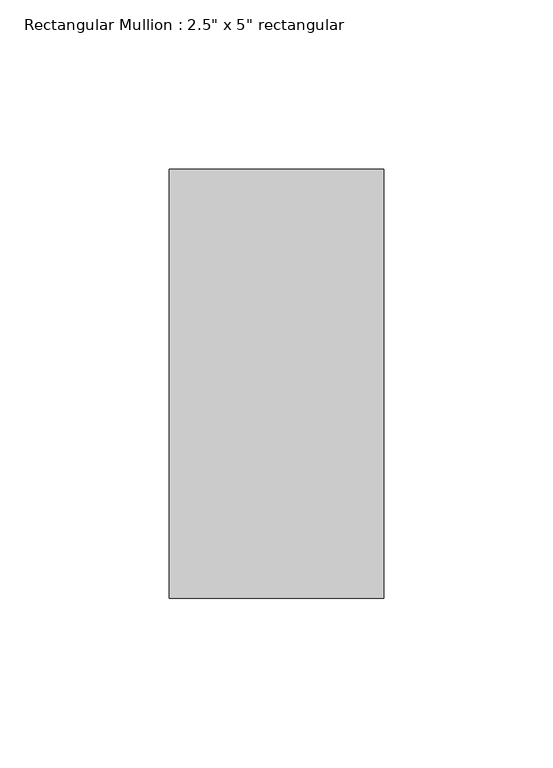
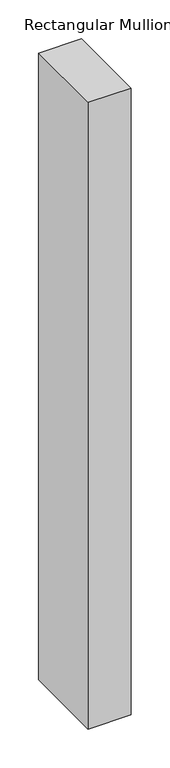
"""IFC4 building model written with IfcOpenShell, lengths in millimetres: member geometry."""

from ifc_helpers import new_model, si_unit, frame, origin, place, context, project, spatial, polyline, outline, extrude, source, transform, mapped, element, save


def member_1093a910(model_context):
    return source(origin(), model_context, "Body", "SweptSolid", [
        extrude(outline(polyline([(0.0, 63.5), (0.0, -63.5), (-63.5, -63.5), (-63.5, 63.5), (0.0, 63.5)])), frame((0.0, 0.0, -982.6547408), z_axis=(0.0, 0.0, 1.0), x_axis=(1.0, 0.0, 0.0)), (0.0, 0.0, 1.0), 982.6547408),
    ])


if __name__ == "__main__":
    model = new_model("IFC4")
    model_context = context("Model", 3, world=origin())
    ifc_project = project(units=[si_unit("LENGTHUNIT", "METRE", prefix="MILLI")], contexts=[model_context])
    site = spatial("IfcSite", under=ifc_project)
    building = spatial("IfcBuilding", under=site)
    placement = place(None, origin())
    member_shape = member_1093a910(model_context)
    element("IfcMember", 1, ObjectType="Rectangular Mullion : 2.5\" x 5\" rectangular", at=placement, inside=building, context=model_context, shape_type="MappedRepresentation", body=[
        mapped(member_shape, transform((0.0, 0.0, 0.0), x_axis=(1.0, 0.0, 0.0), y_axis=(0.0, 1.0, 0.0), z_axis=(0.0, 0.0, 1.0))),
    ])
    save(model, "model.ifc")

# Revit data of these elements
# Type "Rectangular Mullion : 2.5\" x 5\" rectangular"
#   built-in parameter 1007304 = 0.416667 (stored number, unit not read)
#   built-in parameter 1007301 = 0.104167 (stored number, unit not read)
#   built-in parameter 1007300 = 0.104167 (stored number, unit not read)
